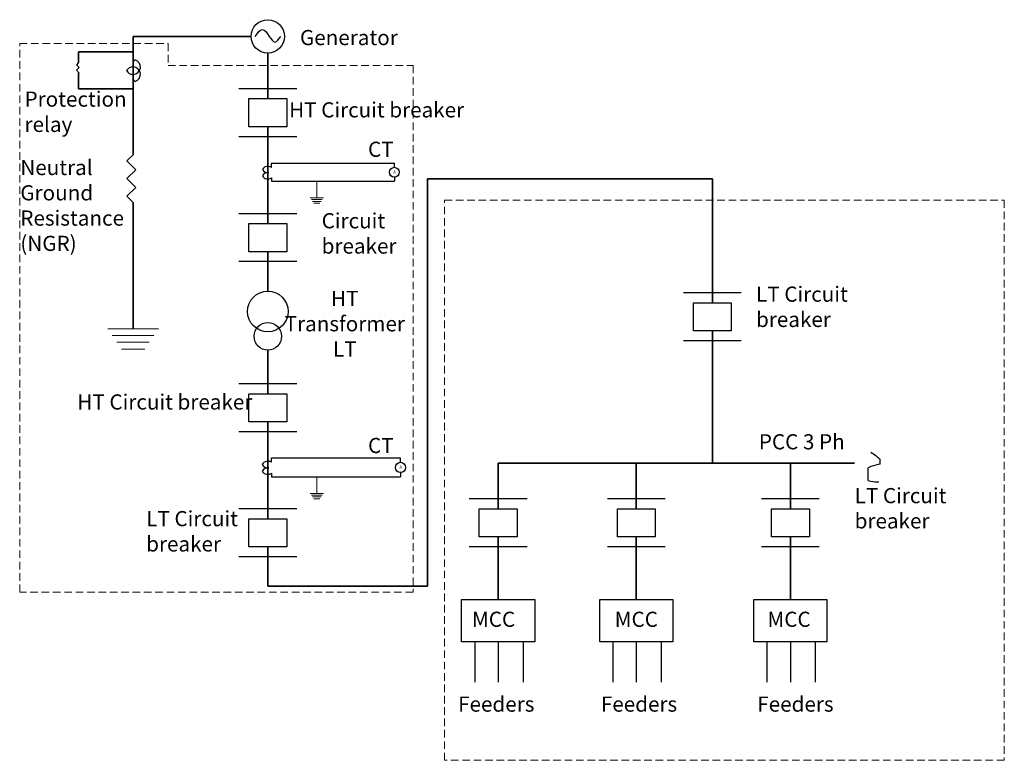
# Model space of a CAD drawing. Units: millimetres. Extents: x 59 to 124, y 27.9 to 76.8.
import ezdxf

# ---------------------------------------------------------------- set-up
doc = ezdxf.new("R2010")
doc.units = ezdxf.units.MM
doc.header["$MEASUREMENT"] = 0
doc.linetypes.add('HIDDENX2', pattern=[0.75, 0.5, -0.25])
for name, color, linetype, lineweight in [('E-ANNO-TEXT', 7, 'Continuous', 18), ('E-ONEL-BNDY', 8, 'HIDDENX2', 18), ('E-ONEL-EQPM', 1, 'Continuous', 25), ('E-ONEL-GRND', 3, 'Continuous', 18), ('E-ONEL-WIRE', 7, 'Continuous', 35)]:
    doc.layers.add(name, color=color, linetype=linetype, lineweight=lineweight)
doc.styles.get("Standard").update_dxf_attribs({"font": 'arial.ttf'})

# ---------------------------------------------------------------- blocks, each defined once
blk = doc.blocks.new('CB-SYMBOL')
for p, q in [((73.474, 72.241), (77.285, 72.241)), ((73.474, 69.084), (77.285, 69.084))]:
    blk.add_line(p, q)
blk.add_lwpolyline([(74.131, 71.573), (76.629, 71.573), (76.629, 69.714), (74.131, 69.714)], close=True)
blk = doc.blocks.new('MCC-PANEL')
for p, q in [((89.028, 35.745), (89.028, 33.095)), ((90.577, 35.745), (90.577, 33.095)), ((92.217, 35.745), (92.217, 33.095))]:
    blk.add_line(p, q)
blk.add_lwpolyline([(88.167, 38.547), (92.987, 38.547), (92.987, 35.745), (88.167, 35.745)], close=True)
blk = doc.blocks.new('GROUND-SYMBOL')
for p, q in [((78.614, 46.631), (78.614, 45.539)), ((78.614, 45.539), (78.175, 45.539)), ((78.614, 45.539), (79.053, 45.539)), ((78.254, 45.422), (78.974, 45.422)), ((78.333, 45.305), (78.894, 45.305)), ((78.413, 45.188), (78.815, 45.188))]:
    blk.add_line(p, q)

msp = doc.modelspace()

# ---------------------------------------------------------------- linework, layer by layer
at = {"layer": 'E-ONEL-BNDY'}
for p, q in [((59.013, 75.205), (68.799, 75.205)), ((59.013, 39.035), (59.013, 75.205)), ((68.799, 75.205), (68.799, 73.75)), ((68.799, 73.75), (84.96, 73.75)), ((84.96, 73.75), (84.96, 39.035)), ((84.96, 39.035), (59.013, 39.035))]:
    msp.add_line(p, q, dxfattribs=at)
msp.add_lwpolyline([(87.033, 64.875), (123.964, 64.875), (123.964, 27.944), (87.033, 27.944)], close=True, dxfattribs=at)
at = {"layer": 'E-ONEL-EQPM'}
for p, q in [((66.629, 74.13), (66.49, 73.992)), ((62.901, 73.953), (62.753, 73.805)), ((62.753, 73.805), (62.937, 73.622)), ((62.937, 73.622), (62.753, 73.438)), ((62.753, 73.438), (62.937, 73.255)), ((62.937, 73.255), (62.901, 73.219)), ((66.629, 72.699), (66.49, 72.838)), ((66.49, 67.865), (66.085, 67.46)), ((66.085, 67.46), (66.667, 66.877)), ((75.613, 67.036), (75.613, 67.31)), ((75.613, 67.31), (83.731, 67.31)), ((83.731, 67.04), (83.731, 67.31)), ((66.667, 66.877), (66.085, 66.295)), ((66.085, 66.295), (66.667, 65.713)), ((75.613, 66.347), (75.613, 66.121)), ((83.731, 66.393), (83.731, 66.121)), ((66.667, 65.713), (66.085, 65.131)), ((75.613, 66.121), (83.731, 66.121)), ((66.085, 65.131), (66.49, 64.725)), ((75.626, 47.591), (75.626, 47.878)), ((75.626, 47.878), (84.135, 47.878)), ((84.135, 47.595), (84.135, 47.878)), ((115.771, 47.476), (115.771, 47.791)), ((75.626, 46.869), (75.626, 46.631)), ((84.135, 46.917), (84.135, 46.631)), ((114.982, 46.395), (114.982, 47.225)), ((75.626, 46.631), (84.135, 46.631))]:
    msp.add_line(p, q, dxfattribs=at)
for centre, radius in [((75.38, 75.673), 1.102), ((83.731, 66.717), 0.324), ((75.38, 57.539), 1.341), ((75.381, 55.899), 0.908), ((84.135, 47.256), 0.339)]:
    msp.add_circle(centre, radius, dxfattribs=at)
for centre, radius, start, end in [((66.49, 73.66), 0.49, 270, 73.55559), ((66.49, 73.17), 0.49, 90, 150), ((66.49, 73.66), 0.49, 210, 270), ((66.49, 73.17), 0.49, 286.44441, 90), ((75.38, 66.691), 0.416, 55.89882, 150), ((75.38, 67.107), 0.416, 210, 278.36608), ((75.38, 66.276), 0.416, 81.63392, 150), ((75.38, 66.691), 0.416, 210, 304.10118), ((75.381, 47.23), 0.436, 55.89882, 150), ((75.381, 47.666), 0.436, 210, 278.36608), ((75.381, 46.794), 0.436, 81.63392, 150), ((75.381, 47.23), 0.436, 210, 304.10118)]:
    msp.add_arc(centre, radius, start, end, dxfattribs=at)
for points, knots in [([(74.556, 75.673), (74.709, 75.903), (75.016, 76.364), (75.448, 75.715), (75.852, 75.111), (76.106, 75.485), (76.234, 75.673)], [0, 0, 0, 0, 0.651184, 1.302369, 1.832526, 2.368454, 2.368454, 2.368454, 2.368454]), ([(115.771, 47.476), (115.628, 47.426), (115.321, 47.384), (115.039, 47.256), (114.982, 47.225)], [1.233378, 1.233378, 1.233378, 1.233378, 1.7831342, 1.9333183, 1.9333183, 1.9333183, 1.9333183]), ([(114.982, 46.395), (115.041, 46.375), (115.297, 46.305), (115.522, 46.3), (115.686, 46.311)], [3.1804154, 3.1804154, 3.1804154, 3.1804154, 3.3391803, 3.8481775, 3.8481775, 3.8481775, 3.8481775])]:
    msp.add_open_spline(points, degree=3, knots=knots, dxfattribs=at)
msp.add_open_spline([(115.161, 48.268), (115.396, 48.099), (115.632, 47.93), (115.771, 47.791)], degree=3, dxfattribs=at)
at = {"layer": 'E-ONEL-GRND'}
for p, q in [((66.49, 56.397), (64.817, 56.397)), ((65.119, 55.951), (67.862, 55.951)), ((66.49, 56.397), (68.164, 56.397)), ((65.421, 55.505), (67.56, 55.505)), ((65.723, 55.059), (67.258, 55.059))]:
    msp.add_line(p, q, dxfattribs=at)
at = {"layer": 'E-ONEL-WIRE'}
for p, q in [((74.278, 75.673), (66.49, 75.673)), ((66.49, 75.673), (66.49, 67.865)), ((66.49, 74.65), (62.901, 74.65)), ((62.901, 74.65), (62.901, 73.953)), ((75.38, 74.571), (75.38, 71.573)), ((62.901, 73.219), (62.901, 72.208)), ((66.49, 72.838), (66.49, 72.208)), ((66.49, 72.208), (62.901, 72.208)), ((75.38, 69.714), (75.38, 63.335)), ((85.914, 39.418), (85.914, 66.289)), ((85.914, 66.289), (104.705, 66.289)), ((104.705, 66.289), (104.705, 63.291)), ((104.705, 66.289), (104.705, 58.117)), ((66.49, 64.725), (66.49, 56.397)), ((75.38, 61.475), (75.38, 58.88)), ((104.705, 56.257), (104.705, 49.16)), ((75.381, 54.992), (75.381, 52.112)), ((75.381, 50.252), (75.381, 43.873)), ((104.705, 49.16), (104.705, 47.527)), ((90.577, 47.527), (114.092, 47.527)), ((90.577, 47.527), (90.577, 44.529)), ((99.69, 47.527), (99.69, 44.529)), ((109.855, 47.527), (109.855, 44.529)), ((90.577, 42.669), (90.577, 38.547)), ((99.69, 42.669), (99.69, 38.547)), ((109.855, 42.669), (109.855, 38.547)), ((75.381, 42.013), (75.381, 39.418)), ((75.381, 39.418), (85.914, 39.418))]:
    msp.add_line(p, q, dxfattribs=at)

# ---------------------------------------------------------------- block references
at = {"layer": 'E-ONEL-EQPM'}
for name, p in [('CB-SYMBOL', (0, 0)), ('CB-SYMBOL', (0, -8.239)), ('CB-SYMBOL', (29.325, -13.457)), ('CB-SYMBOL', (0.002, -19.462)), ('CB-SYMBOL', (15.197, -27.044)), ('CB-SYMBOL', (24.31, -27.044)), ('CB-SYMBOL', (34.475, -27.044)), ('CB-SYMBOL', (0.002, -27.701)), ('MCC-PANEL', (0, 0)), ('MCC-PANEL', (9.113, 0)), ('MCC-PANEL', (19.278, 0))]:
    msp.add_blockref(name, p, dxfattribs=at)
at = {"layer": 'E-ONEL-GRND'}
for p in [(0, 19.489), (0, 0)]:
    msp.add_blockref('GROUND-SYMBOL', p, dxfattribs=at)

# ---------------------------------------------------------------- texts
at = {"layer": 'E-ANNO-TEXT', "attachment_point": 1}
for s, width, insert, char_height in [('Generator', 5.39126, (77.502, 76.098), 1), ('Protection relay', 10.05158, (59.333, 72.04), 1), ('HT Circuit breaker', 12.0839, (76.786, 71.331), 1), ('CT', 5.39126, (81.99, 68.732), 1), ('Neutral\\PGround\\PResistance\\P(NGR)', 5.39126, (59.055, 67.529), 1), ('A', 0.37352, (83.665, 66.844), 0.2), ('Circuit\\Pbreaker', 5.39126, (78.932, 64.019), 1), ('LT Circuit \\Pbreaker', 8.07388, (107.587, 59.18), 1), ('\\pxqc;HT\\PTransformer\\PLT', 5.39126, (77.763, 58.895), 1), ('HT Circuit breaker', 11.99722, (62.817, 52.071), 1), ('PCC 3 Ph', 6.89848, (107.77, 49.446), 1), ('CT', 5.39126, (81.99, 49.2), 1), ('A', 0.37352, (84.069, 47.383), 0.2), ('LT Circuit \\Pbreaker', 8.07388, (114.093, 45.895), 1), ('LT Circuit \\Pbreaker', 8.07388, (67.358, 44.378), 1), ('MCC', 5.39126, (88.847, 37.742), 1), ('MCC', 5.39126, (98.264, 37.742), 1), ('MCC', 5.39126, (108.339, 37.742), 1), ('Feeders', 5.39126, (87.932, 32.15), 1), ('Feeders', 5.39126, (97.35, 32.15), 1), ('Feeders', 5.39126, (107.667, 32.15), 1)]:
    msp.add_mtext_dynamic_manual_height_columns(s, width=width, gutter_width=1, heights=[0], dxfattribs=dict(at, insert=insert, char_height=char_height))

doc.saveas('drawing.dxf')
